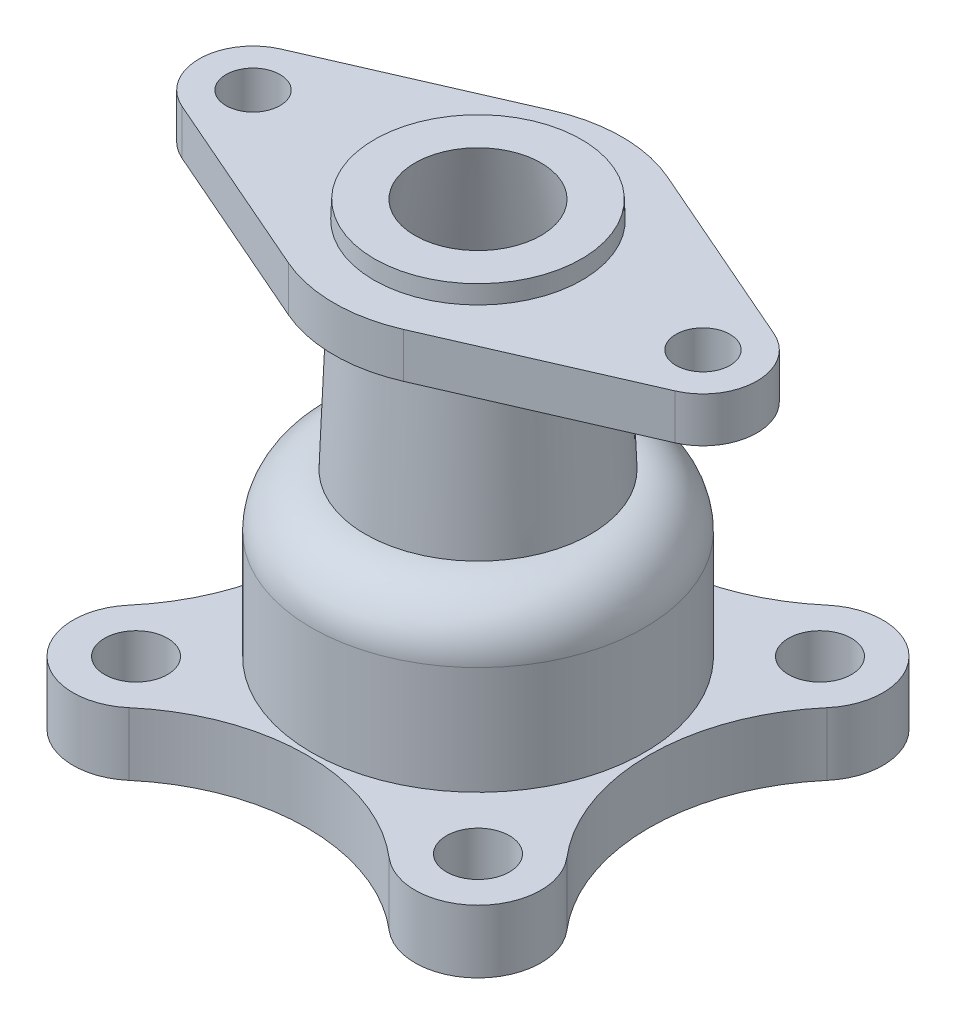
ISO-10303-21;
HEADER;
FILE_DESCRIPTION(('STEP AP214'),'2;1');
FILE_NAME('part.step','',(''),(''),'','','');
FILE_SCHEMA(('AUTOMOTIVE_DESIGN { 1 0 10303 214 1 1 1 1 }'));
ENDSEC;
DATA;
#1=APPLICATION_CONTEXT('core data for automotive mechanical design processes');
#2=APPLICATION_PROTOCOL_DEFINITION('international standard','automotive_design',2000,#1);
#3=PRODUCT_CONTEXT('',#1,'mechanical');
#4=PRODUCT('Part','Part','',(#3));
#5=PRODUCT_RELATED_PRODUCT_CATEGORY('part','',(#4));
#6=PRODUCT_DEFINITION_FORMATION('','',#4);
#7=PRODUCT_DEFINITION_CONTEXT('part definition',#1,'design');
#8=PRODUCT_DEFINITION('design','',#6,#7);
#9=PRODUCT_DEFINITION_SHAPE('','',#8);
#10=(LENGTH_UNIT() NAMED_UNIT(*) SI_UNIT(.MILLI.,.METRE.));
#11=(NAMED_UNIT(*) PLANE_ANGLE_UNIT() SI_UNIT($,.RADIAN.));
#12=(NAMED_UNIT(*) SI_UNIT($,.STERADIAN.) SOLID_ANGLE_UNIT());
#13=UNCERTAINTY_MEASURE_WITH_UNIT(LENGTH_MEASURE(1.E-05),#10,'distance_accuracy_value','');
#14=(GEOMETRIC_REPRESENTATION_CONTEXT(3) GLOBAL_UNCERTAINTY_ASSIGNED_CONTEXT((#13)) GLOBAL_UNIT_ASSIGNED_CONTEXT((#10,
#11,#12)) REPRESENTATION_CONTEXT('',''));
#15=CARTESIAN_POINT('',(0.,0.,0.));
#16=DIRECTION('',(0.,0.,1.));
#17=DIRECTION('',(1.,0.,0.));
#18=AXIS2_PLACEMENT_3D('',#15,#16,#17);
#19=CARTESIAN_POINT('',(0.,102.,0.));
#20=DIRECTION('',(0.,-1.,0.));
#21=DIRECTION('',(0.,0.,-1.));
#22=AXIS2_PLACEMENT_3D('',#19,#20,#21);
#23=CONICAL_SURFACE('',#22,23.,0.038442590021188);
#24=CARTESIAN_POINT('',(0.,50.,0.));
#25=DIRECTION('',(0.,1.,0.));
#26=DIRECTION('',(-0.195132737944331,0.,0.980776842397061));
#27=AXIS2_PLACEMENT_3D('',#24,#25,#26);
#28=CIRCLE('',#27,25.);
#29=CARTESIAN_POINT('',(-4.87831844860826,50.,24.5194210599265));
#30=VERTEX_POINT('',#29);
#31=EDGE_CURVE('E222',#30,#30,#28,.T.);
#32=ORIENTED_EDGE('',*,*,#31,.T.);
#33=EDGE_LOOP('',(#32));
#34=FACE_BOUND('',#33,.T.);
#35=CARTESIAN_POINT('',(0.,88.,0.));
#36=DIRECTION('',(0.,1.,0.));
#37=DIRECTION('',(0.,0.,1.));
#38=AXIS2_PLACEMENT_3D('',#35,#36,#37);
#39=CIRCLE('',#38,23.5384615384615);
#40=CARTESIAN_POINT('',(0.,88.,23.5384615384615));
#41=VERTEX_POINT('',#40);
#42=EDGE_CURVE('E327',#41,#41,#39,.F.);
#43=ORIENTED_EDGE('',*,*,#42,.T.);
#44=EDGE_LOOP('',(#43));
#45=FACE_BOUND('',#44,.T.);
#46=ADVANCED_FACE('F63',(#34,#45),#23,.T.);
#47=CARTESIAN_POINT('',(-38.,14.,-38.));
#48=DIRECTION('',(0.,-1.,0.));
#49=DIRECTION('',(0.,0.,-1.));
#50=AXIS2_PLACEMENT_3D('',#47,#48,#49);
#51=CYLINDRICAL_SURFACE('',#50,14.);
#52=CARTESIAN_POINT('',(-38.,0.,-38.));
#53=DIRECTION('',(0.,1.,0.));
#54=DIRECTION('',(0.,0.,1.));
#55=AXIS2_PLACEMENT_3D('',#52,#53,#54);
#56=CIRCLE('',#55,14.);
#57=CARTESIAN_POINT('',(-28.9170731707317,0.,-48.6536585365853));
#58=VERTEX_POINT('',#57);
#59=CARTESIAN_POINT('',(-48.6536585365854,0.,-28.9170731707319));
#60=VERTEX_POINT('',#59);
#61=EDGE_CURVE('E181',#58,#60,#56,.T.);
#62=ORIENTED_EDGE('',*,*,#61,.T.);
#63=DIRECTION('',(0.,-1.,0.));
#64=VECTOR('',#63,1.);
#65=CARTESIAN_POINT('',(-48.6536585365854,14.,-28.9170731707319));
#66=LINE('',#65,#64);
#67=CARTESIAN_POINT('',(-48.6536585365854,14.,-28.9170731707319));
#68=VERTEX_POINT('',#67);
#69=EDGE_CURVE('E221',#68,#60,#66,.T.);
#70=ORIENTED_EDGE('',*,*,#69,.F.);
#71=CARTESIAN_POINT('',(-38.,14.,-38.));
#72=DIRECTION('',(0.,1.,0.));
#73=DIRECTION('',(0.,0.,1.));
#74=AXIS2_PLACEMENT_3D('',#71,#72,#73);
#75=CIRCLE('',#74,14.);
#76=CARTESIAN_POINT('',(-28.9170731707317,14.,-48.6536585365853));
#77=VERTEX_POINT('',#76);
#78=EDGE_CURVE('E125',#77,#68,#75,.T.);
#79=ORIENTED_EDGE('',*,*,#78,.F.);
#80=DIRECTION('',(0.,-1.,0.));
#81=VECTOR('',#80,1.);
#82=CARTESIAN_POINT('',(-28.9170731707317,14.,-48.6536585365853));
#83=LINE('',#82,#81);
#84=EDGE_CURVE('E85',#77,#58,#83,.T.);
#85=ORIENTED_EDGE('',*,*,#84,.T.);
#86=EDGE_LOOP('',(#62,#70,#79,#85));
#87=FACE_BOUND('',#86,.T.);
#88=ADVANCED_FACE('F254',(#87),#51,.T.);
#89=CARTESIAN_POINT('',(-82.5714285714285,14.,-8.50408930670025E-13));
#90=DIRECTION('',(0.,-1.,0.));
#91=DIRECTION('',(0.,0.,-1.));
#92=AXIS2_PLACEMENT_3D('',#89,#90,#91);
#93=CYLINDRICAL_SURFACE('',#92,44.5714285714285);
#94=CARTESIAN_POINT('',(-82.5714285714285,0.,-8.50408930670025E-13));
#95=DIRECTION('',(0.,1.,0.));
#96=DIRECTION('',(0.,0.,1.));
#97=AXIS2_PLACEMENT_3D('',#94,#95,#96);
#98=CIRCLE('',#97,44.5714285714285);
#99=CARTESIAN_POINT('',(-48.6536585365853,0.,28.9170731707315));
#100=VERTEX_POINT('',#99);
#101=EDGE_CURVE('E183',#100,#60,#98,.T.);
#102=ORIENTED_EDGE('',*,*,#101,.F.);
#103=DIRECTION('',(0.,-1.,0.));
#104=VECTOR('',#103,1.);
#105=CARTESIAN_POINT('',(-48.6536585365853,14.,28.9170731707315));
#106=LINE('',#105,#104);
#107=CARTESIAN_POINT('',(-48.6536585365853,14.,28.9170731707315));
#108=VERTEX_POINT('',#107);
#109=EDGE_CURVE('E217',#108,#100,#106,.T.);
#110=ORIENTED_EDGE('',*,*,#109,.F.);
#111=CARTESIAN_POINT('',(-82.5714285714285,14.,-8.50408930670025E-13));
#112=DIRECTION('',(0.,1.,0.));
#113=DIRECTION('',(0.,0.,1.));
#114=AXIS2_PLACEMENT_3D('',#111,#112,#113);
#115=CIRCLE('',#114,44.5714285714285);
#116=EDGE_CURVE('E340',#108,#68,#115,.T.);
#117=ORIENTED_EDGE('',*,*,#116,.T.);
#118=ORIENTED_EDGE('',*,*,#69,.T.);
#119=EDGE_LOOP('',(#102,#110,#117,#118));
#120=FACE_BOUND('',#119,.T.);
#121=ADVANCED_FACE('F257',(#120),#93,.F.);
#122=CARTESIAN_POINT('',(-38.,14.,38.));
#123=DIRECTION('',(0.,-1.,0.));
#124=DIRECTION('',(0.,0.,-1.));
#125=AXIS2_PLACEMENT_3D('',#122,#123,#124);
#126=CYLINDRICAL_SURFACE('',#125,14.);
#127=CARTESIAN_POINT('',(-38.,0.,38.));
#128=DIRECTION('',(0.,1.,0.));
#129=DIRECTION('',(0.,0.,1.));
#130=AXIS2_PLACEMENT_3D('',#127,#128,#129);
#131=CIRCLE('',#130,14.);
#132=CARTESIAN_POINT('',(-28.9170731707311,0.,48.6536585365849));
#133=VERTEX_POINT('',#132);
#134=EDGE_CURVE('E190',#100,#133,#131,.T.);
#135=ORIENTED_EDGE('',*,*,#134,.T.);
#136=DIRECTION('',(0.,-1.,0.));
#137=VECTOR('',#136,1.);
#138=CARTESIAN_POINT('',(-28.9170731707311,14.,48.6536585365849));
#139=LINE('',#138,#137);
#140=CARTESIAN_POINT('',(-28.9170731707311,14.,48.6536585365849));
#141=VERTEX_POINT('',#140);
#142=EDGE_CURVE('E220',#141,#133,#139,.T.);
#143=ORIENTED_EDGE('',*,*,#142,.F.);
#144=CARTESIAN_POINT('',(-38.,14.,38.));
#145=DIRECTION('',(0.,1.,0.));
#146=DIRECTION('',(0.,0.,1.));
#147=AXIS2_PLACEMENT_3D('',#144,#145,#146);
#148=CIRCLE('',#147,14.);
#149=EDGE_CURVE('E338',#108,#141,#148,.T.);
#150=ORIENTED_EDGE('',*,*,#149,.F.);
#151=ORIENTED_EDGE('',*,*,#109,.T.);
#152=EDGE_LOOP('',(#135,#143,#150,#151));
#153=FACE_BOUND('',#152,.T.);
#154=ADVANCED_FACE('F256',(#153),#126,.T.);
#155=CARTESIAN_POINT('',(2.78280328563949E-12,14.,82.5714285714269));
#156=DIRECTION('',(0.,-1.,0.));
#157=DIRECTION('',(0.,0.,-1.));
#158=AXIS2_PLACEMENT_3D('',#155,#156,#157);
#159=CYLINDRICAL_SURFACE('',#158,44.5714285714285);
#160=CARTESIAN_POINT('',(2.78280328563949E-12,0.,82.5714285714269));
#161=DIRECTION('',(0.,1.,0.));
#162=DIRECTION('',(0.,0.,1.));
#163=AXIS2_PLACEMENT_3D('',#160,#161,#162);
#164=CIRCLE('',#163,44.5714285714285);
#165=CARTESIAN_POINT('',(28.9170731707321,0.,48.6536585365852));
#166=VERTEX_POINT('',#165);
#167=EDGE_CURVE('E188',#166,#133,#164,.T.);
#168=ORIENTED_EDGE('',*,*,#167,.F.);
#169=DIRECTION('',(0.,-1.,0.));
#170=VECTOR('',#169,1.);
#171=CARTESIAN_POINT('',(28.9170731707321,14.,48.6536585365852));
#172=LINE('',#171,#170);
#173=CARTESIAN_POINT('',(28.9170731707321,14.,48.6536585365852));
#174=VERTEX_POINT('',#173);
#175=EDGE_CURVE('E213',#174,#166,#172,.T.);
#176=ORIENTED_EDGE('',*,*,#175,.F.);
#177=CARTESIAN_POINT('',(2.78280328563949E-12,14.,82.5714285714269));
#178=DIRECTION('',(0.,1.,0.));
#179=DIRECTION('',(0.,0.,1.));
#180=AXIS2_PLACEMENT_3D('',#177,#178,#179);
#181=CIRCLE('',#180,44.5714285714285);
#182=EDGE_CURVE('E165',#174,#141,#181,.T.);
#183=ORIENTED_EDGE('',*,*,#182,.T.);
#184=ORIENTED_EDGE('',*,*,#142,.T.);
#185=EDGE_LOOP('',(#168,#176,#183,#184));
#186=FACE_BOUND('',#185,.T.);
#187=ADVANCED_FACE('F263',(#186),#159,.F.);
#188=CARTESIAN_POINT('',(38.,14.,38.));
#189=DIRECTION('',(0.,-1.,0.));
#190=DIRECTION('',(0.,0.,-1.));
#191=AXIS2_PLACEMENT_3D('',#188,#189,#190);
#192=CYLINDRICAL_SURFACE('',#191,14.);
#193=CARTESIAN_POINT('',(38.,0.,38.));
#194=DIRECTION('',(0.,1.,0.));
#195=DIRECTION('',(0.,0.,1.));
#196=AXIS2_PLACEMENT_3D('',#193,#194,#195);
#197=CIRCLE('',#196,14.);
#198=CARTESIAN_POINT('',(48.6536585365856,0.,28.9170731707319));
#199=VERTEX_POINT('',#198);
#200=EDGE_CURVE('E194',#166,#199,#197,.T.);
#201=ORIENTED_EDGE('',*,*,#200,.T.);
#202=DIRECTION('',(0.,-1.,0.));
#203=VECTOR('',#202,1.);
#204=CARTESIAN_POINT('',(48.6536585365856,14.,28.9170731707319));
#205=LINE('',#204,#203);
#206=CARTESIAN_POINT('',(48.6536585365856,14.,28.9170731707319));
#207=VERTEX_POINT('',#206);
#208=EDGE_CURVE('E151',#207,#199,#205,.T.);
#209=ORIENTED_EDGE('',*,*,#208,.F.);
#210=CARTESIAN_POINT('',(38.,14.,38.));
#211=DIRECTION('',(0.,1.,0.));
#212=DIRECTION('',(0.,0.,1.));
#213=AXIS2_PLACEMENT_3D('',#210,#211,#212);
#214=CIRCLE('',#213,14.);
#215=EDGE_CURVE('E163',#174,#207,#214,.T.);
#216=ORIENTED_EDGE('',*,*,#215,.F.);
#217=ORIENTED_EDGE('',*,*,#175,.T.);
#218=EDGE_LOOP('',(#201,#209,#216,#217));
#219=FACE_BOUND('',#218,.T.);
#220=ADVANCED_FACE('F270',(#219),#192,.T.);
#221=CARTESIAN_POINT('',(82.5714285714313,14.,-7.77057947081979E-13));
#222=DIRECTION('',(0.,-1.,0.));
#223=DIRECTION('',(0.,0.,-1.));
#224=AXIS2_PLACEMENT_3D('',#221,#222,#223);
#225=CYLINDRICAL_SURFACE('',#224,44.5714285714306);
#226=CARTESIAN_POINT('',(82.5714285714313,0.,-7.77057947081979E-13));
#227=DIRECTION('',(0.,1.,0.));
#228=DIRECTION('',(0.,0.,1.));
#229=AXIS2_PLACEMENT_3D('',#226,#227,#228);
#230=CIRCLE('',#229,44.5714285714306);
#231=CARTESIAN_POINT('',(48.6536585365857,0.,-28.9170731707322));
#232=VERTEX_POINT('',#231);
#233=EDGE_CURVE('E149',#232,#199,#230,.T.);
#234=ORIENTED_EDGE('',*,*,#233,.F.);
#235=DIRECTION('',(0.,-1.,0.));
#236=VECTOR('',#235,1.);
#237=CARTESIAN_POINT('',(48.6536585365857,14.,-28.9170731707322));
#238=LINE('',#237,#236);
#239=CARTESIAN_POINT('',(48.6536585365857,14.,-28.9170731707322));
#240=VERTEX_POINT('',#239);
#241=EDGE_CURVE('E145',#240,#232,#238,.T.);
#242=ORIENTED_EDGE('',*,*,#241,.F.);
#243=CARTESIAN_POINT('',(82.5714285714313,14.,-7.77057947081979E-13));
#244=DIRECTION('',(0.,1.,0.));
#245=DIRECTION('',(0.,0.,1.));
#246=AXIS2_PLACEMENT_3D('',#243,#244,#245);
#247=CIRCLE('',#246,44.5714285714306);
#248=EDGE_CURVE('E147',#240,#207,#247,.T.);
#249=ORIENTED_EDGE('',*,*,#248,.T.);
#250=ORIENTED_EDGE('',*,*,#208,.T.);
#251=EDGE_LOOP('',(#234,#242,#249,#250));
#252=FACE_BOUND('',#251,.T.);
#253=ADVANCED_FACE('F144',(#252),#225,.F.);
#254=CARTESIAN_POINT('',(38.,14.,-38.));
#255=DIRECTION('',(0.,-1.,0.));
#256=DIRECTION('',(0.,0.,-1.));
#257=AXIS2_PLACEMENT_3D('',#254,#255,#256);
#258=CYLINDRICAL_SURFACE('',#257,14.);
#259=CARTESIAN_POINT('',(38.,0.,-38.));
#260=DIRECTION('',(0.,1.,0.));
#261=DIRECTION('',(0.,0.,1.));
#262=AXIS2_PLACEMENT_3D('',#259,#260,#261);
#263=CIRCLE('',#262,14.);
#264=CARTESIAN_POINT('',(28.9170731707317,0.,-48.6536585365853));
#265=VERTEX_POINT('',#264);
#266=EDGE_CURVE('E200',#232,#265,#263,.T.);
#267=ORIENTED_EDGE('',*,*,#266,.T.);
#268=DIRECTION('',(0.,-1.,0.));
#269=VECTOR('',#268,1.);
#270=CARTESIAN_POINT('',(28.9170731707317,14.,-48.6536585365853));
#271=LINE('',#270,#269);
#272=CARTESIAN_POINT('',(28.9170731707317,14.,-48.6536585365853));
#273=VERTEX_POINT('',#272);
#274=EDGE_CURVE('E109',#273,#265,#271,.T.);
#275=ORIENTED_EDGE('',*,*,#274,.F.);
#276=CARTESIAN_POINT('',(38.,14.,-38.));
#277=DIRECTION('',(0.,1.,0.));
#278=DIRECTION('',(0.,0.,1.));
#279=AXIS2_PLACEMENT_3D('',#276,#277,#278);
#280=CIRCLE('',#279,14.);
#281=EDGE_CURVE('E153',#240,#273,#280,.T.);
#282=ORIENTED_EDGE('',*,*,#281,.F.);
#283=ORIENTED_EDGE('',*,*,#241,.T.);
#284=EDGE_LOOP('',(#267,#275,#282,#283));
#285=FACE_BOUND('',#284,.T.);
#286=ADVANCED_FACE('F152',(#285),#258,.T.);
#287=CARTESIAN_POINT('',(38.,14.,38.));
#288=DIRECTION('',(0.,-1.,0.));
#289=DIRECTION('',(0.,0.,-1.));
#290=AXIS2_PLACEMENT_3D('',#287,#288,#289);
#291=CYLINDRICAL_SURFACE('',#290,7.);
#292=CARTESIAN_POINT('',(38.,14.,38.));
#293=DIRECTION('',(0.,1.,0.));
#294=DIRECTION('',(0.,0.,1.));
#295=AXIS2_PLACEMENT_3D('',#292,#293,#294);
#296=CIRCLE('',#295,7.);
#297=CARTESIAN_POINT('',(38.,14.,45.));
#298=VERTEX_POINT('',#297);
#299=EDGE_CURVE('E175',#298,#298,#296,.T.);
#300=ORIENTED_EDGE('',*,*,#299,.T.);
#301=EDGE_LOOP('',(#300));
#302=FACE_BOUND('',#301,.T.);
#303=CARTESIAN_POINT('',(38.,0.,38.));
#304=DIRECTION('',(0.,1.,0.));
#305=DIRECTION('',(0.,0.,1.));
#306=AXIS2_PLACEMENT_3D('',#303,#304,#305);
#307=CIRCLE('',#306,7.);
#308=CARTESIAN_POINT('',(38.,0.,45.));
#309=VERTEX_POINT('',#308);
#310=EDGE_CURVE('E204',#309,#309,#307,.T.);
#311=ORIENTED_EDGE('',*,*,#310,.F.);
#312=EDGE_LOOP('',(#311));
#313=FACE_BOUND('',#312,.T.);
#314=ADVANCED_FACE('F277',(#302,#313),#291,.F.);
#315=CARTESIAN_POINT('',(38.,14.,-38.));
#316=DIRECTION('',(0.,-1.,0.));
#317=DIRECTION('',(0.,0.,-1.));
#318=AXIS2_PLACEMENT_3D('',#315,#316,#317);
#319=CYLINDRICAL_SURFACE('',#318,7.);
#320=CARTESIAN_POINT('',(38.,14.,-38.));
#321=DIRECTION('',(0.,1.,0.));
#322=DIRECTION('',(0.,0.,1.));
#323=AXIS2_PLACEMENT_3D('',#320,#321,#322);
#324=CIRCLE('',#323,7.);
#325=CARTESIAN_POINT('',(38.,14.,-31.));
#326=VERTEX_POINT('',#325);
#327=EDGE_CURVE('E169',#326,#326,#324,.T.);
#328=ORIENTED_EDGE('',*,*,#327,.T.);
#329=EDGE_LOOP('',(#328));
#330=FACE_BOUND('',#329,.T.);
#331=CARTESIAN_POINT('',(38.,0.,-38.));
#332=DIRECTION('',(0.,1.,0.));
#333=DIRECTION('',(0.,0.,1.));
#334=AXIS2_PLACEMENT_3D('',#331,#332,#333);
#335=CIRCLE('',#334,7.);
#336=CARTESIAN_POINT('',(38.,0.,-31.));
#337=VERTEX_POINT('',#336);
#338=EDGE_CURVE('E205',#337,#337,#335,.T.);
#339=ORIENTED_EDGE('',*,*,#338,.F.);
#340=EDGE_LOOP('',(#339));
#341=FACE_BOUND('',#340,.T.);
#342=ADVANCED_FACE('F276',(#330,#341),#319,.F.);
#343=CARTESIAN_POINT('',(0.,14.,-82.5714285714285));
#344=DIRECTION('',(0.,-1.,0.));
#345=DIRECTION('',(0.,0.,-1.));
#346=AXIS2_PLACEMENT_3D('',#343,#344,#345);
#347=CYLINDRICAL_SURFACE('',#346,44.5714285714285);
#348=CARTESIAN_POINT('',(0.,0.,-82.5714285714285));
#349=DIRECTION('',(0.,1.,0.));
#350=DIRECTION('',(0.,0.,1.));
#351=AXIS2_PLACEMENT_3D('',#348,#349,#350);
#352=CIRCLE('',#351,44.5714285714285);
#353=EDGE_CURVE('E197',#58,#265,#352,.T.);
#354=ORIENTED_EDGE('',*,*,#353,.F.);
#355=ORIENTED_EDGE('',*,*,#84,.F.);
#356=CARTESIAN_POINT('',(0.,14.,-82.5714285714285));
#357=DIRECTION('',(0.,1.,0.));
#358=DIRECTION('',(0.,0.,1.));
#359=AXIS2_PLACEMENT_3D('',#356,#357,#358);
#360=CIRCLE('',#359,44.5714285714285);
#361=EDGE_CURVE('E154',#77,#273,#360,.T.);
#362=ORIENTED_EDGE('',*,*,#361,.T.);
#363=ORIENTED_EDGE('',*,*,#274,.T.);
#364=EDGE_LOOP('',(#354,#355,#362,#363));
#365=FACE_BOUND('',#364,.T.);
#366=ADVANCED_FACE('F252',(#365),#347,.F.);
#367=CARTESIAN_POINT('',(-38.,14.,-38.));
#368=DIRECTION('',(0.,-1.,0.));
#369=DIRECTION('',(0.,0.,-1.));
#370=AXIS2_PLACEMENT_3D('',#367,#368,#369);
#371=CYLINDRICAL_SURFACE('',#370,7.);
#372=CARTESIAN_POINT('',(-38.,14.,-38.));
#373=DIRECTION('',(0.,1.,0.));
#374=DIRECTION('',(0.,0.,1.));
#375=AXIS2_PLACEMENT_3D('',#372,#373,#374);
#376=CIRCLE('',#375,7.);
#377=CARTESIAN_POINT('',(-38.,14.,-31.));
#378=VERTEX_POINT('',#377);
#379=EDGE_CURVE('E212',#378,#378,#376,.T.);
#380=ORIENTED_EDGE('',*,*,#379,.T.);
#381=EDGE_LOOP('',(#380));
#382=FACE_BOUND('',#381,.T.);
#383=CARTESIAN_POINT('',(-38.,0.,-38.));
#384=DIRECTION('',(0.,1.,0.));
#385=DIRECTION('',(0.,0.,1.));
#386=AXIS2_PLACEMENT_3D('',#383,#384,#385);
#387=CIRCLE('',#386,7.);
#388=CARTESIAN_POINT('',(-38.,0.,-31.));
#389=VERTEX_POINT('',#388);
#390=EDGE_CURVE('E178',#389,#389,#387,.T.);
#391=ORIENTED_EDGE('',*,*,#390,.F.);
#392=EDGE_LOOP('',(#391));
#393=FACE_BOUND('',#392,.T.);
#394=ADVANCED_FACE('F250',(#382,#393),#371,.F.);
#395=CARTESIAN_POINT('',(-38.,14.,38.));
#396=DIRECTION('',(0.,-1.,0.));
#397=DIRECTION('',(0.,0.,-1.));
#398=AXIS2_PLACEMENT_3D('',#395,#396,#397);
#399=CYLINDRICAL_SURFACE('',#398,7.);
#400=CARTESIAN_POINT('',(-38.,14.,38.));
#401=DIRECTION('',(0.,1.,0.));
#402=DIRECTION('',(0.,0.,1.));
#403=AXIS2_PLACEMENT_3D('',#400,#401,#402);
#404=CIRCLE('',#403,7.);
#405=CARTESIAN_POINT('',(-38.,14.,45.));
#406=VERTEX_POINT('',#405);
#407=EDGE_CURVE('E174',#406,#406,#404,.T.);
#408=ORIENTED_EDGE('',*,*,#407,.T.);
#409=EDGE_LOOP('',(#408));
#410=FACE_BOUND('',#409,.T.);
#411=CARTESIAN_POINT('',(-38.,0.,38.));
#412=DIRECTION('',(0.,1.,0.));
#413=DIRECTION('',(0.,0.,1.));
#414=AXIS2_PLACEMENT_3D('',#411,#412,#413);
#415=CIRCLE('',#414,7.);
#416=CARTESIAN_POINT('',(-38.,0.,45.));
#417=VERTEX_POINT('',#416);
#418=EDGE_CURVE('E206',#417,#417,#415,.T.);
#419=ORIENTED_EDGE('',*,*,#418,.F.);
#420=EDGE_LOOP('',(#419));
#421=FACE_BOUND('',#420,.T.);
#422=ADVANCED_FACE('F249',(#410,#421),#399,.F.);
#423=CARTESIAN_POINT('',(0.,14.,0.));
#424=DIRECTION('',(0.,1.,0.));
#425=DIRECTION('',(0.,0.,1.));
#426=AXIS2_PLACEMENT_3D('',#423,#424,#425);
#427=PLANE('',#426);
#428=CARTESIAN_POINT('',(0.,14.,0.));
#429=DIRECTION('',(0.,1.,0.));
#430=DIRECTION('',(0.,0.,1.));
#431=AXIS2_PLACEMENT_3D('',#428,#429,#430);
#432=CIRCLE('',#431,37.);
#433=CARTESIAN_POINT('',(0.,14.,37.));
#434=VERTEX_POINT('',#433);
#435=EDGE_CURVE('E185',#434,#434,#432,.T.);
#436=ORIENTED_EDGE('',*,*,#435,.F.);
#437=EDGE_LOOP('',(#436));
#438=FACE_BOUND('',#437,.T.);
#439=ORIENTED_EDGE('',*,*,#379,.F.);
#440=EDGE_LOOP('',(#439));
#441=FACE_BOUND('',#440,.T.);
#442=ORIENTED_EDGE('',*,*,#78,.T.);
#443=ORIENTED_EDGE('',*,*,#116,.F.);
#444=ORIENTED_EDGE('',*,*,#149,.T.);
#445=ORIENTED_EDGE('',*,*,#182,.F.);
#446=ORIENTED_EDGE('',*,*,#215,.T.);
#447=ORIENTED_EDGE('',*,*,#248,.F.);
#448=ORIENTED_EDGE('',*,*,#281,.T.);
#449=ORIENTED_EDGE('',*,*,#361,.F.);
#450=EDGE_LOOP('',(#442,#443,#444,#445,#446,#447,#448,#449));
#451=FACE_BOUND('',#450,.T.);
#452=ORIENTED_EDGE('',*,*,#327,.F.);
#453=EDGE_LOOP('',(#452));
#454=FACE_BOUND('',#453,.T.);
#455=ORIENTED_EDGE('',*,*,#299,.F.);
#456=EDGE_LOOP('',(#455));
#457=FACE_BOUND('',#456,.T.);
#458=ORIENTED_EDGE('',*,*,#407,.F.);
#459=EDGE_LOOP('',(#458));
#460=FACE_BOUND('',#459,.T.);
#461=ADVANCED_FACE('F160',(#438,#441,#451,#454,#457,#460),#427,.T.);
#462=CARTESIAN_POINT('',(0.,0.,0.));
#463=DIRECTION('',(0.,1.,0.));
#464=DIRECTION('',(0.,0.,1.));
#465=AXIS2_PLACEMENT_3D('',#462,#463,#464);
#466=PLANE('',#465);
#467=CARTESIAN_POINT('',(0.,0.,0.));
#468=DIRECTION('',(0.,-1.,0.));
#469=DIRECTION('',(0.,0.,-1.));
#470=AXIS2_PLACEMENT_3D('',#467,#468,#469);
#471=CIRCLE('',#470,30.);
#472=CARTESIAN_POINT('',(0.,0.,-30.));
#473=VERTEX_POINT('',#472);
#474=EDGE_CURVE('E378',#473,#473,#471,.T.);
#475=ORIENTED_EDGE('',*,*,#474,.F.);
#476=EDGE_LOOP('',(#475));
#477=FACE_BOUND('',#476,.T.);
#478=ORIENTED_EDGE('',*,*,#390,.T.);
#479=EDGE_LOOP('',(#478));
#480=FACE_BOUND('',#479,.T.);
#481=ORIENTED_EDGE('',*,*,#61,.F.);
#482=ORIENTED_EDGE('',*,*,#353,.T.);
#483=ORIENTED_EDGE('',*,*,#266,.F.);
#484=ORIENTED_EDGE('',*,*,#233,.T.);
#485=ORIENTED_EDGE('',*,*,#200,.F.);
#486=ORIENTED_EDGE('',*,*,#167,.T.);
#487=ORIENTED_EDGE('',*,*,#134,.F.);
#488=ORIENTED_EDGE('',*,*,#101,.T.);
#489=EDGE_LOOP('',(#481,#482,#483,#484,#485,#486,#487,#488));
#490=FACE_BOUND('',#489,.T.);
#491=ORIENTED_EDGE('',*,*,#338,.T.);
#492=EDGE_LOOP('',(#491));
#493=FACE_BOUND('',#492,.T.);
#494=ORIENTED_EDGE('',*,*,#310,.T.);
#495=EDGE_LOOP('',(#494));
#496=FACE_BOUND('',#495,.T.);
#497=ORIENTED_EDGE('',*,*,#418,.T.);
#498=EDGE_LOOP('',(#497));
#499=FACE_BOUND('',#498,.T.);
#500=ADVANCED_FACE('F288',(#477,#480,#490,#493,#496,#499),#466,.F.);
#501=CARTESIAN_POINT('',(0.,50.,0.));
#502=DIRECTION('',(0.,-1.,0.));
#503=DIRECTION('',(0.,0.,-1.));
#504=AXIS2_PLACEMENT_3D('',#501,#502,#503);
#505=CYLINDRICAL_SURFACE('',#504,37.);
#506=CARTESIAN_POINT('',(0.,38.,0.));
#507=DIRECTION('',(0.,1.,0.));
#508=DIRECTION('',(0.,0.,1.));
#509=AXIS2_PLACEMENT_3D('',#506,#507,#508);
#510=CIRCLE('',#509,37.);
#511=CARTESIAN_POINT('',(0.,38.,37.));
#512=VERTEX_POINT('',#511);
#513=EDGE_CURVE('E223',#512,#512,#510,.F.);
#514=ORIENTED_EDGE('',*,*,#513,.T.);
#515=EDGE_LOOP('',(#514));
#516=FACE_BOUND('',#515,.T.);
#517=ORIENTED_EDGE('',*,*,#435,.T.);
#518=EDGE_LOOP('',(#517));
#519=FACE_BOUND('',#518,.T.);
#520=ADVANCED_FACE('F244',(#516,#519),#505,.T.);
#521=CARTESIAN_POINT('',(0.,38.,0.));
#522=DIRECTION('',(0.,1.,0.));
#523=DIRECTION('',(0.,0.,1.));
#524=AXIS2_PLACEMENT_3D('',#521,#522,#523);
#525=TOROIDAL_SURFACE('',#524,25.,12.);
#526=ORIENTED_EDGE('',*,*,#513,.F.);
#527=EDGE_LOOP('',(#526));
#528=FACE_BOUND('',#527,.T.);
#529=ORIENTED_EDGE('',*,*,#31,.F.);
#530=EDGE_LOOP('',(#529));
#531=FACE_BOUND('',#530,.T.);
#532=ADVANCED_FACE('F232',(#528,#531),#525,.T.);
#533=CARTESIAN_POINT('',(12.8,88.,-29.3284844477174));
#534=DIRECTION('',(0.4,0.,-0.916515138991168));
#535=DIRECTION('',(-0.916515138991168,0.,-0.4));
#536=AXIS2_PLACEMENT_3D('',#533,#534,#535);
#537=PLANE('',#536);
#538=DIRECTION('',(-0.916515138991168,0.,-0.4));
#539=VECTOR('',#538,1.);
#540=CARTESIAN_POINT('',(12.8,98.,-29.3284844477174));
#541=LINE('',#540,#539);
#542=CARTESIAN_POINT('',(54.8,98.,-10.998181667894));
#543=VERTEX_POINT('',#542);
#544=CARTESIAN_POINT('',(12.8,98.,-29.3284844477174));
#545=VERTEX_POINT('',#544);
#546=EDGE_CURVE('E395',#543,#545,#541,.T.);
#547=ORIENTED_EDGE('',*,*,#546,.F.);
#548=DIRECTION('',(0.,1.,0.));
#549=VECTOR('',#548,1.);
#550=CARTESIAN_POINT('',(54.8,88.,-10.998181667894));
#551=LINE('',#550,#549);
#552=CARTESIAN_POINT('',(54.8,88.,-10.998181667894));
#553=VERTEX_POINT('',#552);
#554=EDGE_CURVE('E370',#553,#543,#551,.T.);
#555=ORIENTED_EDGE('',*,*,#554,.F.);
#556=DIRECTION('',(-0.916515138991168,0.,-0.4));
#557=VECTOR('',#556,1.);
#558=CARTESIAN_POINT('',(12.8,88.,-29.3284844477174));
#559=LINE('',#558,#557);
#560=CARTESIAN_POINT('',(12.8,88.,-29.3284844477174));
#561=VERTEX_POINT('',#560);
#562=EDGE_CURVE('E393',#553,#561,#559,.T.);
#563=ORIENTED_EDGE('',*,*,#562,.T.);
#564=DIRECTION('',(0.,1.,0.));
#565=VECTOR('',#564,1.);
#566=CARTESIAN_POINT('',(12.8,88.,-29.3284844477174));
#567=LINE('',#566,#565);
#568=EDGE_CURVE('E425',#561,#545,#567,.T.);
#569=ORIENTED_EDGE('',*,*,#568,.T.);
#570=EDGE_LOOP('',(#547,#555,#563,#569));
#571=FACE_BOUND('',#570,.T.);
#572=ADVANCED_FACE('F242',(#571),#537,.T.);
#573=CARTESIAN_POINT('',(50.,88.,0.));
#574=DIRECTION('',(0.,1.,0.));
#575=DIRECTION('',(0.,0.,1.));
#576=AXIS2_PLACEMENT_3D('',#573,#574,#575);
#577=CYLINDRICAL_SURFACE('',#576,12.);
#578=CARTESIAN_POINT('',(50.,98.,0.));
#579=DIRECTION('',(0.,1.,0.));
#580=DIRECTION('',(0.,0.,1.));
#581=AXIS2_PLACEMENT_3D('',#578,#579,#580);
#582=CIRCLE('',#581,12.);
#583=CARTESIAN_POINT('',(54.8,98.,10.998181667894));
#584=VERTEX_POINT('',#583);
#585=EDGE_CURVE('E444',#584,#543,#582,.T.);
#586=ORIENTED_EDGE('',*,*,#585,.F.);
#587=DIRECTION('',(0.,1.,0.));
#588=VECTOR('',#587,1.);
#589=CARTESIAN_POINT('',(54.8,88.,10.998181667894));
#590=LINE('',#589,#588);
#591=CARTESIAN_POINT('',(54.8,88.,10.998181667894));
#592=VERTEX_POINT('',#591);
#593=EDGE_CURVE('E371',#592,#584,#590,.T.);
#594=ORIENTED_EDGE('',*,*,#593,.F.);
#595=CARTESIAN_POINT('',(50.,88.,0.));
#596=DIRECTION('',(0.,1.,0.));
#597=DIRECTION('',(0.,0.,1.));
#598=AXIS2_PLACEMENT_3D('',#595,#596,#597);
#599=CIRCLE('',#598,12.);
#600=EDGE_CURVE('E414',#592,#553,#599,.T.);
#601=ORIENTED_EDGE('',*,*,#600,.T.);
#602=ORIENTED_EDGE('',*,*,#554,.T.);
#603=EDGE_LOOP('',(#586,#594,#601,#602));
#604=FACE_BOUND('',#603,.T.);
#605=ADVANCED_FACE('F484',(#604),#577,.T.);
#606=CARTESIAN_POINT('',(12.8,88.,29.3284844477174));
#607=DIRECTION('',(-0.4,0.,-0.916515138991168));
#608=DIRECTION('',(-0.916515138991168,0.,0.4));
#609=AXIS2_PLACEMENT_3D('',#606,#607,#608);
#610=PLANE('',#609);
#611=DIRECTION('',(-0.916515138991168,0.,0.4));
#612=VECTOR('',#611,1.);
#613=CARTESIAN_POINT('',(12.8,98.,29.3284844477174));
#614=LINE('',#613,#612);
#615=CARTESIAN_POINT('',(12.8,98.,29.3284844477174));
#616=VERTEX_POINT('',#615);
#617=EDGE_CURVE('E445',#584,#616,#614,.T.);
#618=ORIENTED_EDGE('',*,*,#617,.T.);
#619=DIRECTION('',(0.,1.,0.));
#620=VECTOR('',#619,1.);
#621=CARTESIAN_POINT('',(12.8,88.,29.3284844477174));
#622=LINE('',#621,#620);
#623=CARTESIAN_POINT('',(12.8,88.,29.3284844477174));
#624=VERTEX_POINT('',#623);
#625=EDGE_CURVE('E453',#624,#616,#622,.T.);
#626=ORIENTED_EDGE('',*,*,#625,.F.);
#627=DIRECTION('',(-0.916515138991168,0.,0.4));
#628=VECTOR('',#627,1.);
#629=CARTESIAN_POINT('',(12.8,88.,29.3284844477174));
#630=LINE('',#629,#628);
#631=EDGE_CURVE('E415',#592,#624,#630,.T.);
#632=ORIENTED_EDGE('',*,*,#631,.F.);
#633=ORIENTED_EDGE('',*,*,#593,.T.);
#634=EDGE_LOOP('',(#618,#626,#632,#633));
#635=FACE_BOUND('',#634,.T.);
#636=ADVANCED_FACE('F491',(#635),#610,.F.);
#637=CARTESIAN_POINT('',(0.,88.,0.));
#638=DIRECTION('',(0.,1.,0.));
#639=DIRECTION('',(0.,0.,1.));
#640=AXIS2_PLACEMENT_3D('',#637,#638,#639);
#641=CYLINDRICAL_SURFACE('',#640,32.);
#642=CARTESIAN_POINT('',(0.,98.,0.));
#643=DIRECTION('',(0.,1.,0.));
#644=DIRECTION('',(0.,0.,1.));
#645=AXIS2_PLACEMENT_3D('',#642,#643,#644);
#646=CIRCLE('',#645,32.);
#647=CARTESIAN_POINT('',(-12.8,98.,29.3284844477174));
#648=VERTEX_POINT('',#647);
#649=EDGE_CURVE('E437',#648,#616,#646,.T.);
#650=ORIENTED_EDGE('',*,*,#649,.F.);
#651=DIRECTION('',(0.,1.,0.));
#652=VECTOR('',#651,1.);
#653=CARTESIAN_POINT('',(-12.8,88.,29.3284844477174));
#654=LINE('',#653,#652);
#655=CARTESIAN_POINT('',(-12.8,88.,29.3284844477174));
#656=VERTEX_POINT('',#655);
#657=EDGE_CURVE('E458',#656,#648,#654,.T.);
#658=ORIENTED_EDGE('',*,*,#657,.F.);
#659=CARTESIAN_POINT('',(0.,88.,0.));
#660=DIRECTION('',(0.,1.,0.));
#661=DIRECTION('',(0.,0.,1.));
#662=AXIS2_PLACEMENT_3D('',#659,#660,#661);
#663=CIRCLE('',#662,32.);
#664=EDGE_CURVE('E406',#656,#624,#663,.T.);
#665=ORIENTED_EDGE('',*,*,#664,.T.);
#666=ORIENTED_EDGE('',*,*,#625,.T.);
#667=EDGE_LOOP('',(#650,#658,#665,#666));
#668=FACE_BOUND('',#667,.T.);
#669=ADVANCED_FACE('F505',(#668),#641,.T.);
#670=CARTESIAN_POINT('',(-12.8,88.,29.3284844477174));
#671=DIRECTION('',(-0.4,0.,0.916515138991168));
#672=DIRECTION('',(0.916515138991168,0.,0.4));
#673=AXIS2_PLACEMENT_3D('',#670,#671,#672);
#674=PLANE('',#673);
#675=DIRECTION('',(0.916515138991168,0.,0.4));
#676=VECTOR('',#675,1.);
#677=CARTESIAN_POINT('',(-12.8,98.,29.3284844477174));
#678=LINE('',#677,#676);
#679=CARTESIAN_POINT('',(-54.8,98.,10.998181667894));
#680=VERTEX_POINT('',#679);
#681=EDGE_CURVE('E436',#680,#648,#678,.T.);
#682=ORIENTED_EDGE('',*,*,#681,.F.);
#683=DIRECTION('',(0.,1.,0.));
#684=VECTOR('',#683,1.);
#685=CARTESIAN_POINT('',(-54.8,88.,10.998181667894));
#686=LINE('',#685,#684);
#687=CARTESIAN_POINT('',(-54.8,88.,10.998181667894));
#688=VERTEX_POINT('',#687);
#689=EDGE_CURVE('E461',#688,#680,#686,.T.);
#690=ORIENTED_EDGE('',*,*,#689,.F.);
#691=DIRECTION('',(0.916515138991168,0.,0.4));
#692=VECTOR('',#691,1.);
#693=CARTESIAN_POINT('',(-12.8,88.,29.3284844477174));
#694=LINE('',#693,#692);
#695=EDGE_CURVE('E407',#688,#656,#694,.T.);
#696=ORIENTED_EDGE('',*,*,#695,.T.);
#697=ORIENTED_EDGE('',*,*,#657,.T.);
#698=EDGE_LOOP('',(#682,#690,#696,#697));
#699=FACE_BOUND('',#698,.T.);
#700=ADVANCED_FACE('F512',(#699),#674,.T.);
#701=CARTESIAN_POINT('',(-50.,88.,0.));
#702=DIRECTION('',(0.,1.,0.));
#703=DIRECTION('',(0.,0.,1.));
#704=AXIS2_PLACEMENT_3D('',#701,#702,#703);
#705=CYLINDRICAL_SURFACE('',#704,12.);
#706=CARTESIAN_POINT('',(-50.,98.,0.));
#707=DIRECTION('',(0.,1.,0.));
#708=DIRECTION('',(0.,0.,1.));
#709=AXIS2_PLACEMENT_3D('',#706,#707,#708);
#710=CIRCLE('',#709,12.);
#711=CARTESIAN_POINT('',(-54.8,98.,-10.998181667894));
#712=VERTEX_POINT('',#711);
#713=EDGE_CURVE('E433',#712,#680,#710,.T.);
#714=ORIENTED_EDGE('',*,*,#713,.F.);
#715=DIRECTION('',(0.,1.,0.));
#716=VECTOR('',#715,1.);
#717=CARTESIAN_POINT('',(-54.8,88.,-10.998181667894));
#718=LINE('',#717,#716);
#719=CARTESIAN_POINT('',(-54.8,88.,-10.998181667894));
#720=VERTEX_POINT('',#719);
#721=EDGE_CURVE('E463',#720,#712,#718,.T.);
#722=ORIENTED_EDGE('',*,*,#721,.F.);
#723=CARTESIAN_POINT('',(-50.,88.,0.));
#724=DIRECTION('',(0.,1.,0.));
#725=DIRECTION('',(0.,0.,1.));
#726=AXIS2_PLACEMENT_3D('',#723,#724,#725);
#727=CIRCLE('',#726,12.);
#728=EDGE_CURVE('E401',#720,#688,#727,.T.);
#729=ORIENTED_EDGE('',*,*,#728,.T.);
#730=ORIENTED_EDGE('',*,*,#689,.T.);
#731=EDGE_LOOP('',(#714,#722,#729,#730));
#732=FACE_BOUND('',#731,.T.);
#733=ADVANCED_FACE('F518',(#732),#705,.T.);
#734=CARTESIAN_POINT('',(-12.8,88.,-29.3284844477174));
#735=DIRECTION('',(0.4,0.,0.916515138991168));
#736=DIRECTION('',(0.916515138991168,0.,-0.4));
#737=AXIS2_PLACEMENT_3D('',#734,#735,#736);
#738=PLANE('',#737);
#739=DIRECTION('',(0.916515138991168,0.,-0.4));
#740=VECTOR('',#739,1.);
#741=CARTESIAN_POINT('',(-12.8,98.,-29.3284844477174));
#742=LINE('',#741,#740);
#743=CARTESIAN_POINT('',(-12.8,98.,-29.3284844477174));
#744=VERTEX_POINT('',#743);
#745=EDGE_CURVE('E427',#712,#744,#742,.T.);
#746=ORIENTED_EDGE('',*,*,#745,.T.);
#747=DIRECTION('',(0.,1.,0.));
#748=VECTOR('',#747,1.);
#749=CARTESIAN_POINT('',(-12.8,88.,-29.3284844477174));
#750=LINE('',#749,#748);
#751=CARTESIAN_POINT('',(-12.8,88.,-29.3284844477174));
#752=VERTEX_POINT('',#751);
#753=EDGE_CURVE('E470',#752,#744,#750,.T.);
#754=ORIENTED_EDGE('',*,*,#753,.F.);
#755=DIRECTION('',(0.916515138991168,0.,-0.4));
#756=VECTOR('',#755,1.);
#757=CARTESIAN_POINT('',(-12.8,88.,-29.3284844477174));
#758=LINE('',#757,#756);
#759=EDGE_CURVE('E399',#720,#752,#758,.T.);
#760=ORIENTED_EDGE('',*,*,#759,.F.);
#761=ORIENTED_EDGE('',*,*,#721,.T.);
#762=EDGE_LOOP('',(#746,#754,#760,#761));
#763=FACE_BOUND('',#762,.T.);
#764=ADVANCED_FACE('F528',(#763),#738,.F.);
#765=CARTESIAN_POINT('',(50.,88.,0.));
#766=DIRECTION('',(0.,1.,0.));
#767=DIRECTION('',(0.,0.,1.));
#768=AXIS2_PLACEMENT_3D('',#765,#766,#767);
#769=CYLINDRICAL_SURFACE('',#768,6.);
#770=CARTESIAN_POINT('',(50.,88.,0.));
#771=DIRECTION('',(0.,1.,0.));
#772=DIRECTION('',(0.,0.,1.));
#773=AXIS2_PLACEMENT_3D('',#770,#771,#772);
#774=CIRCLE('',#773,6.);
#775=CARTESIAN_POINT('',(50.,88.,6.));
#776=VERTEX_POINT('',#775);
#777=EDGE_CURVE('E417',#776,#776,#774,.T.);
#778=ORIENTED_EDGE('',*,*,#777,.F.);
#779=EDGE_LOOP('',(#778));
#780=FACE_BOUND('',#779,.T.);
#781=CARTESIAN_POINT('',(50.,98.,0.));
#782=DIRECTION('',(0.,1.,0.));
#783=DIRECTION('',(0.,0.,1.));
#784=AXIS2_PLACEMENT_3D('',#781,#782,#783);
#785=CIRCLE('',#784,6.);
#786=CARTESIAN_POINT('',(50.,98.,6.));
#787=VERTEX_POINT('',#786);
#788=EDGE_CURVE('E449',#787,#787,#785,.T.);
#789=ORIENTED_EDGE('',*,*,#788,.T.);
#790=EDGE_LOOP('',(#789));
#791=FACE_BOUND('',#790,.T.);
#792=ADVANCED_FACE('F539',(#780,#791),#769,.F.);
#793=CARTESIAN_POINT('',(0.,88.,0.));
#794=DIRECTION('',(0.,1.,0.));
#795=DIRECTION('',(0.,0.,1.));
#796=AXIS2_PLACEMENT_3D('',#793,#794,#795);
#797=CYLINDRICAL_SURFACE('',#796,32.);
#798=CARTESIAN_POINT('',(0.,98.,0.));
#799=DIRECTION('',(0.,1.,0.));
#800=DIRECTION('',(0.,0.,1.));
#801=AXIS2_PLACEMENT_3D('',#798,#799,#800);
#802=CIRCLE('',#801,32.);
#803=EDGE_CURVE('E430',#545,#744,#802,.T.);
#804=ORIENTED_EDGE('',*,*,#803,.F.);
#805=ORIENTED_EDGE('',*,*,#568,.F.);
#806=CARTESIAN_POINT('',(0.,88.,0.));
#807=DIRECTION('',(0.,1.,0.));
#808=DIRECTION('',(0.,0.,1.));
#809=AXIS2_PLACEMENT_3D('',#806,#807,#808);
#810=CIRCLE('',#809,32.);
#811=EDGE_CURVE('E396',#561,#752,#810,.T.);
#812=ORIENTED_EDGE('',*,*,#811,.T.);
#813=ORIENTED_EDGE('',*,*,#753,.T.);
#814=EDGE_LOOP('',(#804,#805,#812,#813));
#815=FACE_BOUND('',#814,.T.);
#816=ADVANCED_FACE('F548',(#815),#797,.T.);
#817=CARTESIAN_POINT('',(-50.,88.,0.));
#818=DIRECTION('',(0.,1.,0.));
#819=DIRECTION('',(0.,0.,1.));
#820=AXIS2_PLACEMENT_3D('',#817,#818,#819);
#821=CYLINDRICAL_SURFACE('',#820,6.);
#822=CARTESIAN_POINT('',(-50.,88.,0.));
#823=DIRECTION('',(0.,1.,0.));
#824=DIRECTION('',(0.,0.,1.));
#825=AXIS2_PLACEMENT_3D('',#822,#823,#824);
#826=CIRCLE('',#825,6.);
#827=CARTESIAN_POINT('',(-50.,88.,6.));
#828=VERTEX_POINT('',#827);
#829=EDGE_CURVE('E423',#828,#828,#826,.T.);
#830=ORIENTED_EDGE('',*,*,#829,.F.);
#831=EDGE_LOOP('',(#830));
#832=FACE_BOUND('',#831,.T.);
#833=CARTESIAN_POINT('',(-50.,98.,0.));
#834=DIRECTION('',(0.,1.,0.));
#835=DIRECTION('',(0.,0.,1.));
#836=AXIS2_PLACEMENT_3D('',#833,#834,#835);
#837=CIRCLE('',#836,6.);
#838=CARTESIAN_POINT('',(-50.,98.,6.));
#839=VERTEX_POINT('',#838);
#840=EDGE_CURVE('E400',#839,#839,#837,.T.);
#841=ORIENTED_EDGE('',*,*,#840,.T.);
#842=EDGE_LOOP('',(#841));
#843=FACE_BOUND('',#842,.T.);
#844=ADVANCED_FACE('F561',(#832,#843),#821,.F.);
#845=CARTESIAN_POINT('',(0.,88.,0.));
#846=DIRECTION('',(0.,1.,0.));
#847=DIRECTION('',(0.,0.,1.));
#848=AXIS2_PLACEMENT_3D('',#845,#846,#847);
#849=PLANE('',#848);
#850=ORIENTED_EDGE('',*,*,#42,.F.);
#851=EDGE_LOOP('',(#850));
#852=FACE_BOUND('',#851,.T.);
#853=ORIENTED_EDGE('',*,*,#562,.F.);
#854=ORIENTED_EDGE('',*,*,#600,.F.);
#855=ORIENTED_EDGE('',*,*,#631,.T.);
#856=ORIENTED_EDGE('',*,*,#664,.F.);
#857=ORIENTED_EDGE('',*,*,#695,.F.);
#858=ORIENTED_EDGE('',*,*,#728,.F.);
#859=ORIENTED_EDGE('',*,*,#759,.T.);
#860=ORIENTED_EDGE('',*,*,#811,.F.);
#861=EDGE_LOOP('',(#853,#854,#855,#856,#857,#858,#859,#860));
#862=FACE_BOUND('',#861,.T.);
#863=ORIENTED_EDGE('',*,*,#777,.T.);
#864=EDGE_LOOP('',(#863));
#865=FACE_BOUND('',#864,.T.);
#866=ORIENTED_EDGE('',*,*,#829,.T.);
#867=EDGE_LOOP('',(#866));
#868=FACE_BOUND('',#867,.T.);
#869=ADVANCED_FACE('F571',(#852,#862,#865,#868),#849,.F.);
#870=CARTESIAN_POINT('',(0.,98.,0.));
#871=DIRECTION('',(0.,1.,0.));
#872=DIRECTION('',(0.,0.,1.));
#873=AXIS2_PLACEMENT_3D('',#870,#871,#872);
#874=PLANE('',#873);
#875=CARTESIAN_POINT('',(0.,98.,0.));
#876=DIRECTION('',(0.,1.,0.));
#877=DIRECTION('',(0.,0.,1.));
#878=AXIS2_PLACEMENT_3D('',#875,#876,#877);
#879=CIRCLE('',#878,23.1538461538461);
#880=CARTESIAN_POINT('',(0.,98.,23.1538461538461));
#881=VERTEX_POINT('',#880);
#882=EDGE_CURVE('E73',#881,#881,#879,.F.);
#883=ORIENTED_EDGE('',*,*,#882,.T.);
#884=EDGE_LOOP('',(#883));
#885=FACE_BOUND('',#884,.T.);
#886=ORIENTED_EDGE('',*,*,#546,.T.);
#887=ORIENTED_EDGE('',*,*,#803,.T.);
#888=ORIENTED_EDGE('',*,*,#745,.F.);
#889=ORIENTED_EDGE('',*,*,#713,.T.);
#890=ORIENTED_EDGE('',*,*,#681,.T.);
#891=ORIENTED_EDGE('',*,*,#649,.T.);
#892=ORIENTED_EDGE('',*,*,#617,.F.);
#893=ORIENTED_EDGE('',*,*,#585,.T.);
#894=EDGE_LOOP('',(#886,#887,#888,#889,#890,#891,#892,#893));
#895=FACE_BOUND('',#894,.T.);
#896=ORIENTED_EDGE('',*,*,#788,.F.);
#897=EDGE_LOOP('',(#896));
#898=FACE_BOUND('',#897,.T.);
#899=ORIENTED_EDGE('',*,*,#840,.F.);
#900=EDGE_LOOP('',(#899));
#901=FACE_BOUND('',#900,.T.);
#902=ADVANCED_FACE('F581',(#885,#895,#898,#901),#874,.T.);
#903=CARTESIAN_POINT('',(0.,102.,0.));
#904=DIRECTION('',(0.,1.,0.));
#905=DIRECTION('',(0.,0.,1.));
#906=AXIS2_PLACEMENT_3D('',#903,#904,#905);
#907=PLANE('',#906);
#908=CARTESIAN_POINT('',(0.,102.,0.));
#909=DIRECTION('',(0.,1.,0.));
#910=DIRECTION('',(0.,0.,1.));
#911=AXIS2_PLACEMENT_3D('',#908,#909,#910);
#912=CIRCLE('',#911,14.);
#913=CARTESIAN_POINT('',(0.,102.,14.));
#914=VERTEX_POINT('',#913);
#915=EDGE_CURVE('E381',#914,#914,#912,.T.);
#916=ORIENTED_EDGE('',*,*,#915,.F.);
#917=EDGE_LOOP('',(#916));
#918=FACE_BOUND('',#917,.T.);
#919=CARTESIAN_POINT('',(0.,102.,0.));
#920=DIRECTION('',(0.,1.,0.));
#921=DIRECTION('',(0.,0.,1.));
#922=AXIS2_PLACEMENT_3D('',#919,#920,#921);
#923=CIRCLE('',#922,23.);
#924=CARTESIAN_POINT('',(0.,102.,23.));
#925=VERTEX_POINT('',#924);
#926=EDGE_CURVE('E322',#925,#925,#923,.T.);
#927=ORIENTED_EDGE('',*,*,#926,.T.);
#928=EDGE_LOOP('',(#927));
#929=FACE_BOUND('',#928,.T.);
#930=ADVANCED_FACE('F302',(#918,#929),#907,.T.);
#931=ORIENTED_EDGE('',*,*,#882,.F.);
#932=EDGE_LOOP('',(#931));
#933=FACE_BOUND('',#932,.T.);
#934=ORIENTED_EDGE('',*,*,#926,.F.);
#935=EDGE_LOOP('',(#934));
#936=FACE_BOUND('',#935,.T.);
#937=ADVANCED_FACE('F299',(#933,#936),#23,.T.);
#938=CARTESIAN_POINT('',(0.,102.,0.));
#939=DIRECTION('',(0.,-1.,0.));
#940=DIRECTION('',(0.,0.,1.));
#941=AXIS2_PLACEMENT_3D('',#938,#939,#940);
#942=CONICAL_SURFACE('',#941,14.,0.191986217719377);
#943=CARTESIAN_POINT('',(0.,52.,0.));
#944=DIRECTION('',(0.,1.,0.));
#945=DIRECTION('',(0.,0.,1.));
#946=AXIS2_PLACEMENT_3D('',#943,#944,#945);
#947=CIRCLE('',#946,23.7190154568859);
#948=CARTESIAN_POINT('',(0.,52.,23.7190154568859));
#949=VERTEX_POINT('',#948);
#950=EDGE_CURVE('E386',#949,#949,#947,.T.);
#951=ORIENTED_EDGE('',*,*,#950,.F.);
#952=EDGE_LOOP('',(#951));
#953=FACE_BOUND('',#952,.T.);
#954=ORIENTED_EDGE('',*,*,#915,.T.);
#955=EDGE_LOOP('',(#954));
#956=FACE_BOUND('',#955,.T.);
#957=ADVANCED_FACE('F303',(#953,#956),#942,.F.);
#958=CARTESIAN_POINT('',(0.,52.,0.));
#959=DIRECTION('',(0.,1.,0.));
#960=DIRECTION('',(0.,0.,1.));
#961=AXIS2_PLACEMENT_3D('',#958,#959,#960);
#962=PLANE('',#961);
#963=CARTESIAN_POINT('',(0.,52.,0.));
#964=DIRECTION('',(0.,1.,0.));
#965=DIRECTION('',(0.,0.,1.));
#966=AXIS2_PLACEMENT_3D('',#963,#964,#965);
#967=CIRCLE('',#966,19.8922239248386);
#968=CARTESIAN_POINT('',(0.,52.,19.8922239248386));
#969=VERTEX_POINT('',#968);
#970=EDGE_CURVE('E374',#969,#969,#967,.T.);
#971=ORIENTED_EDGE('',*,*,#970,.F.);
#972=EDGE_LOOP('',(#971));
#973=FACE_BOUND('',#972,.T.);
#974=ORIENTED_EDGE('',*,*,#950,.T.);
#975=EDGE_LOOP('',(#974));
#976=FACE_BOUND('',#975,.T.);
#977=ADVANCED_FACE('F613',(#973,#976),#962,.T.);
#978=CARTESIAN_POINT('',(0.,40.,0.));
#979=DIRECTION('',(0.,-1.,0.));
#980=DIRECTION('',(0.,0.,-1.));
#981=AXIS2_PLACEMENT_3D('',#978,#979,#980);
#982=CYLINDRICAL_SURFACE('',#981,30.);
#983=CARTESIAN_POINT('',(0.,26.8545656733411,0.));
#984=DIRECTION('',(0.,1.,0.));
#985=DIRECTION('',(0.,0.,1.));
#986=AXIS2_PLACEMENT_3D('',#983,#984,#985);
#987=CIRCLE('',#986,30.);
#988=CARTESIAN_POINT('',(0.,26.8545656733411,30.));
#989=VERTEX_POINT('',#988);
#990=EDGE_CURVE('E12',#989,#989,#987,.T.);
#991=ORIENTED_EDGE('',*,*,#990,.T.);
#992=EDGE_LOOP('',(#991));
#993=FACE_BOUND('',#992,.T.);
#994=ORIENTED_EDGE('',*,*,#474,.T.);
#995=EDGE_LOOP('',(#994));
#996=FACE_BOUND('',#995,.T.);
#997=ADVANCED_FACE('F633',(#993,#996),#982,.F.);
#998=CARTESIAN_POINT('',(0.,0.,0.));
#999=DIRECTION('',(0.,-1.,0.));
#1000=DIRECTION('',(0.,0.,-1.));
#1001=AXIS2_PLACEMENT_3D('',#998,#999,#1000);
#1002=CONICAL_SURFACE('',#1001,30.,0.191986217719377);
#1003=ORIENTED_EDGE('',*,*,#970,.T.);
#1004=EDGE_LOOP('',(#1003));
#1005=FACE_BOUND('',#1004,.T.);
#1006=CARTESIAN_POINT('',(0.,40.,0.));
#1007=DIRECTION('',(0.,-1.,0.));
#1008=DIRECTION('',(0.,0.,-1.));
#1009=AXIS2_PLACEMENT_3D('',#1006,#1007,#1008);
#1010=CIRCLE('',#1009,22.2247876344912);
#1011=CARTESIAN_POINT('',(0.,40.,-22.2247876344912));
#1012=VERTEX_POINT('',#1011);
#1013=EDGE_CURVE('E373',#1012,#1012,#1010,.T.);
#1014=ORIENTED_EDGE('',*,*,#1013,.T.);
#1015=EDGE_LOOP('',(#1014));
#1016=FACE_BOUND('',#1015,.T.);
#1017=ADVANCED_FACE('F645',(#1005,#1016),#1002,.F.);
#1018=CARTESIAN_POINT('',(0.,26.8545656733411,0.));
#1019=DIRECTION('',(0.,1.,0.));
#1020=DIRECTION('',(0.,0.,1.));
#1021=AXIS2_PLACEMENT_3D('',#1018,#1019,#1020);
#1022=DEGENERATE_TOROIDAL_SURFACE('',#1021,15.,15.,.T.);
#1023=ORIENTED_EDGE('',*,*,#990,.F.);
#1024=EDGE_LOOP('',(#1023));
#1025=FACE_BOUND('',#1024,.T.);
#1026=ORIENTED_EDGE('',*,*,#1013,.F.);
#1027=EDGE_LOOP('',(#1026));
#1028=FACE_BOUND('',#1027,.T.);
#1029=ADVANCED_FACE('F70',(#1025,#1028),#1022,.F.);
#1030=CLOSED_SHELL('',(#46,#88,#121,#154,#187,#220,#253,#286,#314,#342,#366,#394,#422,#461,#500,
#520,#532,#572,#605,#636,#669,#700,#733,#764,#792,#816,#844,#869,#902,#930,#937,#957,#977,#997,
#1017,#1029));
#1031=MANIFOLD_SOLID_BREP('B2',#1030);
#1032=ADVANCED_BREP_SHAPE_REPRESENTATION('',(#18,#1031),#14);
#1033=SHAPE_DEFINITION_REPRESENTATION(#9,#1032);
ENDSEC;
END-ISO-10303-21;
